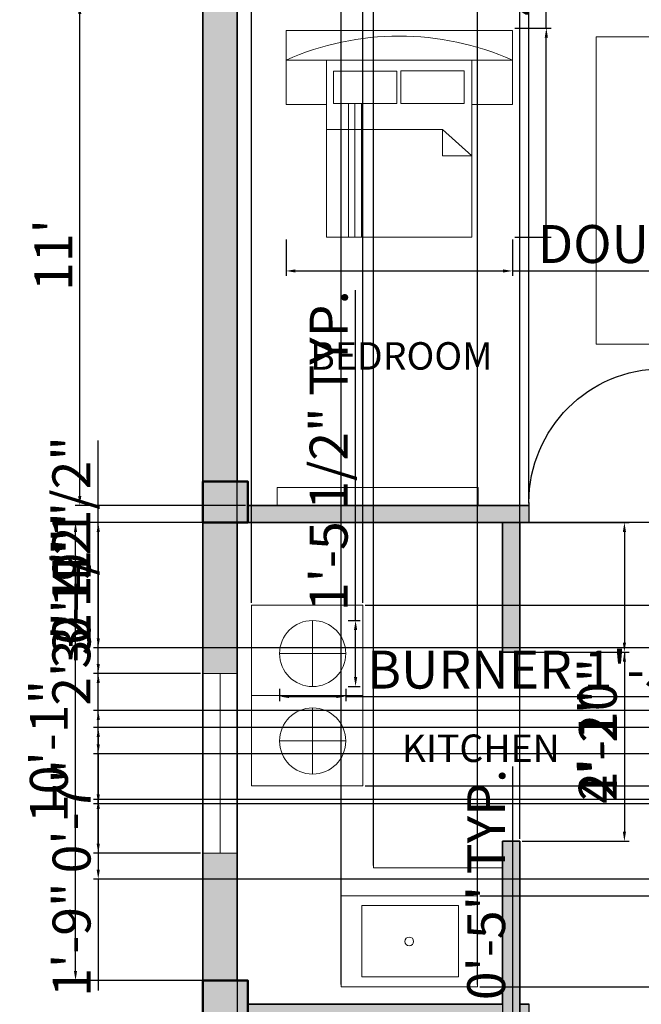
# Model space of a CAD drawing. Units: inches. Extents: x 2312 to 2808, y 1290 to 1909.
# Tile 2 of 5: x 2312 to 2476, y 1503 to 1763. Entities that reach past the tile are written whole.
import ezdxf

# ---------------------------------------------------------------- set-up
doc = ezdxf.new("R2010")
doc.units = ezdxf.units.IN
for name, color, linetype, lineweight in [('A-ANNO-DIMS', 2, 'Continuous', 18), ('A-AREA-IDEN', 7, 'Continuous', 25), ('A-COLS-PATT', 1, 'Continuous', 13), ('A-EQPM', 210, 'Continuous', 18), ('A-FLOR-CASE', 181, 'Continuous', 20), ('A-FLOR-FIXT', 9, 'Continuous', 18), ('A-WALL-PATT', 150, 'Continuous', 13), ('COLUMN', 1, 'Continuous', 50), ('DOOR', 50, 'Continuous', 25), ('FUR', 130, 'Continuous', 18), ('WALL', 7, 'Continuous', 35), ('WINDOW', 70, 'Continuous', 18)]:
    doc.layers.add(name, color=color, linetype=linetype, lineweight=lineweight)
doc.styles.get("Standard").update_dxf_attribs({"font": 'arial.ttf'})
doc.dimstyles.new('ISO-25', dxfattribs={"dimtxt": 10, "dimasz": 2.5, "dimexe": 1.25, "dimexo": 0.625, "dimtad": 1, "dimdec": 0, "dimlunit": 4, "dimtxsty": 'Standard', "dimcen": 2.5, "dimadec": 0, "dimazin": 0, "dimtfac": 1, "dimtdec": 0, "dimtmove": 0, "dimatfit": 3, "dimfxl": 1, "dimarcsym": 0})

# ---------------------------------------------------------------- blocks, each defined once
blk = doc.blocks.new('*U2')
for p, q in [((0, 0), (0, -6)), ((40, 0), (40, -6))]:
    blk.add_line(p, q)
blk.add_lwpolyline([(0, 0), (0, 40), (1.75, 40), (1.75, 0)], close=True)
blk.add_arc((0, 0), 40, 0, 90)
blk = doc.blocks.new('*D20')
at = {"layer": 'A-ANNO-DIMS', "color": 0, "lineweight": -2, "transparency": 16777216}
for p, q in [((2368.81, 1630.22), (2325.59, 1630.22)), ((2326.84, 1511.99), (2326.84, 1627.72)), ((2368.81, 1509.49), (2325.59, 1509.49))]:
    blk.add_line(p, q, dxfattribs=at)
at = {"layer": 'A-ANNO-DIMS', "color": 0, "transparency": 16777216}
for points in [[(2326.42, 1627.72), (2327.25, 1627.72), (2326.84, 1630.22)], [(2326.42, 1511.99), (2327.25, 1511.99), (2326.84, 1509.49)]]:
    blk.add_solid(points, dxfattribs=at)
at = {"layer": 'Defpoints', "color": 0, "transparency": 16777216}
for p in [(2326.84, 1630.22), (2369.43, 1630.22), (2369.43, 1509.49)]:
    blk.add_point(p, dxfattribs=at)
at = {"layer": 'A-ANNO-DIMS', "color": 0, "transparency": 16777216, "insert": (2321.11, 1569.86), "char_height": 10, "attachment_point": 5, "rotation": 90}
blk.add_mtext('10\'-1"', dxfattribs=at)
blk = doc.blocks.new('*D21')
at = {"layer": 'A-ANNO-DIMS', "color": 0, "lineweight": -2, "transparency": 16777216}
for p, q in [((2371.65, 1766.72), (2326.71, 1766.72)), ((2327.96, 1637.22), (2327.96, 1764.22)), ((2371.65, 1634.72), (2326.71, 1634.72))]:
    blk.add_line(p, q, dxfattribs=at)
at = {"layer": 'A-ANNO-DIMS', "color": 0, "transparency": 16777216}
for points in [[(2327.54, 1764.22), (2328.38, 1764.22), (2327.96, 1766.72)], [(2327.54, 1637.22), (2328.38, 1637.22), (2327.96, 1634.72)]]:
    blk.add_solid(points, dxfattribs=at)
at = {"layer": 'Defpoints', "color": 0, "transparency": 16777216}
for p in [(2327.96, 1766.72), (2372.28, 1766.72), (2372.28, 1634.72)]:
    blk.add_point(p, dxfattribs=at)
at = {"layer": 'A-ANNO-DIMS', "color": 0, "transparency": 16777216, "insert": (2322.31, 1700.72), "char_height": 10, "attachment_point": 5, "rotation": 90}
blk.add_mtext("11'", dxfattribs=at)
blk = doc.blocks.new('BED-DOUBLE')
for p, q in [((0, 46.6), (0, 54.42)), ((0, 54.42), (59.67, 54.42)), ((59.67, 54.42), (59.67, 46.6)), ((16.43, 35.15), (16.43, 0)), ((18.15, 35.15), (18.15, 0)), ((19.9, 35.15), (19.9, 0)), ((10.68, 28.37), (10.68, 28.37)), ((10.68, 28.37), (41.23, 28.37)), ((41.23, 28.37), (41.23, 21.43)), ((48.99, 21.43), (41.23, 28.37)), ((41.23, 21.43), (48.99, 21.43))]:
    blk.add_line(p, q)
for points in [[(10.68, 46.6), (0, 46.6), (0, 34.89), (10.68, 34.89)], [(10.68, 46.6), (48.99, 46.6), (48.99, 0), (10.68, 0)], [(59.67, 46.6), (48.99, 46.6), (48.99, 34.89), (59.67, 34.89)], [(12.51, 43.74), (29.18, 43.74), (29.18, 35.15), (12.51, 35.15)], [(30.28, 43.78), (46.95, 43.78), (46.95, 35.19), (30.28, 35.19)]]:
    blk.add_lwpolyline(points, close=True)
blk.add_arc((29.84, -20.26), 73.22, 65.9516, 114.0484)
blk = doc.blocks.new('BEDROOM-STORAGE')
blk.add_lwpolyline([(18.34, 80.97), (0, 80.97), (0, 0), (18.34, 0)], close=True)
blk = doc.blocks.new('BEDROOM-WALL-UNIT')
blk.add_lwpolyline([(0, 0), (52.94, 0), (52.94, 4.76), (0, 4.76)], close=True)
blk = doc.blocks.new('COOKTOP-BURNER')
for p, q in [((8.7, 8.71), (8.7, 17.41)), ((8.7, 17.41), (8.7, 0)), ((0, 8.71), (17.41, 8.71)), ((17.41, 8.71), (8.7, 8.71))]:
    blk.add_line(p, q)
blk.add_circle((8.7, 8.71), 8.71)
blk = doc.blocks.new('*D29')
at = {"layer": 'A-ANNO-DIMS', "color": 0, "lineweight": -2, "transparency": 16777216}
for p, q in [((2382.33, 1704.84), (2382.33, 1695.26)), ((2442, 1704.84), (2442, 1695.26)), ((2384.83, 1696.51), (2439.5, 1696.51)), ((2442, 1696.51), (2631.22, 1696.51))]:
    blk.add_line(p, q, dxfattribs=at)
at = {"layer": 'A-ANNO-DIMS', "color": 0, "transparency": 16777216}
for points in [[(2384.83, 1696.93), (2384.83, 1696.09), (2382.33, 1696.51)], [(2439.5, 1696.93), (2439.5, 1696.09), (2442, 1696.51)]]:
    blk.add_solid(points, dxfattribs=at)
at = {"layer": 'Defpoints', "color": 0, "transparency": 16777216}
for p in [(2382.33, 1705.46), (2442, 1705.46), (2442, 1696.51)]:
    blk.add_point(p, dxfattribs=at)
at = {"layer": 'A-ANNO-DIMS', "color": 0, "transparency": 16777216, "insert": (2537.86, 1702.31), "char_height": 10, "attachment_point": 5}
blk.add_mtext('DOUBLE BED 4\'-11 1/2" TYP.', dxfattribs=at)
blk = doc.blocks.new('*D30')
at = {"layer": 'A-ANNO-DIMS', "color": 0, "lineweight": -2, "transparency": 16777216}
for p, q in [((2450.95, 1760.54), (2450.95, 1825.65)), ((2442.63, 1760.54), (2452.2, 1760.54)), ((2450.95, 1707.96), (2450.95, 1758.04)), ((2442.63, 1705.46), (2452.2, 1705.46))]:
    blk.add_line(p, q, dxfattribs=at)
at = {"layer": 'A-ANNO-DIMS', "color": 0, "transparency": 16777216}
for points in [[(2450.54, 1758.04), (2451.37, 1758.04), (2450.95, 1760.54)], [(2450.54, 1707.96), (2451.37, 1707.96), (2450.95, 1705.46)]]:
    blk.add_solid(points, dxfattribs=at)
at = {"layer": 'Defpoints', "color": 0, "transparency": 16777216}
for p in [(2442, 1760.54), (2450.95, 1760.54), (2442, 1705.46)]:
    blk.add_point(p, dxfattribs=at)
at = {"layer": 'A-ANNO-DIMS', "color": 0, "transparency": 16777216, "insert": (2445.32, 1794.34), "char_height": 10, "attachment_point": 5, "rotation": 90}
blk.add_mtext('4\'-7" TYP.', dxfattribs=at)
blk = doc.blocks.new('*D33')
at = {"layer": 'A-ANNO-DIMS', "color": 0, "lineweight": -2, "transparency": 16777216}
for p, q in [((2381.24, 1493.33), (2381.24, 1484.77)), ((2434.18, 1493.33), (2434.18, 1484.77)), ((2383.74, 1486.02), (2431.68, 1486.02)), ((2434.18, 1486.02), (2577.69, 1486.02))]:
    blk.add_line(p, q, dxfattribs=at)
at = {"layer": 'A-ANNO-DIMS', "color": 0, "transparency": 16777216}
for points in [[(2383.74, 1486.43), (2383.74, 1485.6), (2381.24, 1486.02)], [(2431.68, 1486.43), (2431.68, 1485.6), (2434.18, 1486.02)]]:
    blk.add_solid(points, dxfattribs=at)
at = {"layer": 'Defpoints', "color": 0, "transparency": 16777216}
for p in [(2381.24, 1493.96), (2434.18, 1493.96), (2434.18, 1486.02)]:
    blk.add_point(p, dxfattribs=at)
at = {"layer": 'A-ANNO-DIMS', "color": 0, "transparency": 16777216, "insert": (2507.19, 1491.73), "char_height": 10, "attachment_point": 5}
blk.add_mtext('WALL UNIT 4\'-5" TYP.', dxfattribs=at)
blk = doc.blocks.new('*D34')
at = {"layer": 'A-ANNO-DIMS', "color": 0, "lineweight": -2, "transparency": 16777216}
for p, q in [((2442.12, 1501.22), (2442.12, 1565.92)), ((2434.81, 1498.72), (2443.37, 1498.72)), ((2442.12, 1493.96), (2442.12, 1498.72)), ((2434.81, 1493.96), (2443.37, 1493.96)), ((2442.12, 1491.46), (2442.12, 1488.96))]:
    blk.add_line(p, q, dxfattribs=at)
at = {"layer": 'A-ANNO-DIMS', "color": 0, "transparency": 16777216}
for points in [[(2441.7, 1501.22), (2442.54, 1501.22), (2442.12, 1498.72)], [(2441.7, 1491.46), (2442.54, 1491.46), (2442.12, 1493.96)]]:
    blk.add_solid(points, dxfattribs=at)
at = {"layer": 'Defpoints', "color": 0, "transparency": 16777216}
for p in [(2434.18, 1498.72), (2442.12, 1498.72), (2434.18, 1493.96)]:
    blk.add_point(p, dxfattribs=at)
at = {"layer": 'A-ANNO-DIMS', "color": 0, "transparency": 16777216, "insert": (2436.39, 1534.82), "char_height": 10, "attachment_point": 5, "rotation": 90}
blk.add_mtext('0\'-5" TYP.', dxfattribs=at)
blk = doc.blocks.new('*D37')
at = {"layer": 'A-ANNO-DIMS', "color": 0, "lineweight": -2, "transparency": 16777216}
for p, q in [((2380.65, 1586.33), (2380.65, 1583.1)), ((2398.06, 1586.33), (2398.06, 1583.1)), ((2383.15, 1584.35), (2395.56, 1584.35)), ((2398.06, 1584.35), (2548.49, 1584.35))]:
    blk.add_line(p, q, dxfattribs=at)
at = {"layer": 'A-ANNO-DIMS', "color": 0, "transparency": 16777216}
for points in [[(2383.15, 1584.76), (2383.15, 1583.93), (2380.65, 1584.35)], [(2395.56, 1584.76), (2395.56, 1583.93), (2398.06, 1584.35)]]:
    blk.add_solid(points, dxfattribs=at)
at = {"layer": 'Defpoints', "color": 0, "transparency": 16777216}
for p in [(2380.65, 1586.96), (2398.06, 1586.96), (2398.06, 1584.35)]:
    blk.add_point(p, dxfattribs=at)
at = {"layer": 'A-ANNO-DIMS', "color": 0, "transparency": 16777216, "insert": (2474.53, 1590.14), "char_height": 10, "attachment_point": 5}
blk.add_mtext('BURNER 1\'-5 1/2" TYP.', dxfattribs=at)
blk = doc.blocks.new('*D38')
at = {"layer": 'A-ANNO-DIMS', "color": 0, "lineweight": -2, "transparency": 16777216}
for p, q in [((2400.67, 1604.37), (2400.67, 1691.43)), ((2398.68, 1604.37), (2401.92, 1604.37)), ((2400.67, 1589.46), (2400.67, 1601.87)), ((2398.68, 1586.96), (2401.92, 1586.96))]:
    blk.add_line(p, q, dxfattribs=at)
at = {"layer": 'A-ANNO-DIMS', "color": 0, "transparency": 16777216}
for points in [[(2400.25, 1601.87), (2401.09, 1601.87), (2400.67, 1604.37)], [(2400.25, 1589.46), (2401.09, 1589.46), (2400.67, 1586.96)]]:
    blk.add_solid(points, dxfattribs=at)
at = {"layer": 'Defpoints', "color": 0, "transparency": 16777216}
for p in [(2398.06, 1604.37), (2400.67, 1604.37), (2398.06, 1586.96)]:
    blk.add_point(p, dxfattribs=at)
at = {"layer": 'A-ANNO-DIMS', "color": 0, "transparency": 16777216, "insert": (2394.87, 1649.15), "char_height": 10, "attachment_point": 5, "rotation": 90}
blk.add_mtext('1\'-5 1/2" TYP.', dxfattribs=at)
blk = doc.blocks.new('*D40')
at = {"layer": 'A-ANNO-DIMS', "color": 0, "lineweight": -2, "transparency": 16777216}
for p, q in [((2439.43, 1545.58), (2439.43, 1326.46)), ((2369.43, 1542.44), (2369.43, 1326.46)), ((2371.93, 1327.71), (2436.93, 1327.71))]:
    blk.add_line(p, q, dxfattribs=at)
at = {"layer": 'A-ANNO-DIMS', "color": 0, "transparency": 16777216}
for points in [[(2371.93, 1328.13), (2371.93, 1327.3), (2369.43, 1327.71)], [(2436.93, 1328.13), (2436.93, 1327.3), (2439.43, 1327.71)]]:
    blk.add_solid(points, dxfattribs=at)
at = {"layer": 'Defpoints', "color": 0, "transparency": 16777216}
for p in [(2439.43, 1546.2), (2369.43, 1543.07), (2439.43, 1327.71)]:
    blk.add_point(p, dxfattribs=at)
at = {"layer": 'A-ANNO-DIMS', "color": 0, "transparency": 16777216, "insert": (2404.43, 1333.44), "char_height": 10, "attachment_point": 5}
blk.add_mtext('5\'-10"', dxfattribs=at)
blk = doc.blocks.new('*D41')
at = {"layer": 'A-ANNO-DIMS', "color": 0, "lineweight": -2, "transparency": 16777216}
for p, q in [((2443.93, 1546.83), (2443.93, 1804.57)), ((2482.43, 1510.12), (2482.43, 1804.57)), ((2446.43, 1803.32), (2479.93, 1803.32)), ((2482.43, 1803.32), (2536.06, 1803.32))]:
    blk.add_line(p, q, dxfattribs=at)
at = {"layer": 'A-ANNO-DIMS', "color": 0, "transparency": 16777216}
for points in [[(2446.43, 1803.73), (2446.43, 1802.9), (2443.93, 1803.32)], [(2479.93, 1803.73), (2479.93, 1802.9), (2482.43, 1803.32)]]:
    blk.add_solid(points, dxfattribs=at)
at = {"layer": 'Defpoints', "color": 0, "transparency": 16777216}
for p in [(2482.43, 1803.32), (2443.93, 1546.2), (2482.43, 1509.49)]:
    blk.add_point(p, dxfattribs=at)
at = {"layer": 'A-ANNO-DIMS', "color": 0, "transparency": 16777216, "insert": (2510.5, 1809.12), "char_height": 10, "attachment_point": 5}
blk.add_mtext('3\'-2 1/2"', dxfattribs=at)
blk = doc.blocks.new('*D50')
at = {"layer": 'A-ANNO-DIMS', "color": 0, "lineweight": -2, "transparency": 16777216}
for p, q in [((2446.36, 1635.34), (2446.36, 1804.57)), ((2482.43, 1635.34), (2482.43, 1804.57)), ((2448.86, 1803.32), (2479.93, 1803.32))]:
    blk.add_line(p, q, dxfattribs=at)
at = {"layer": 'A-ANNO-DIMS', "color": 0, "transparency": 16777216}
for points in [[(2448.86, 1803.73), (2448.86, 1802.9), (2446.36, 1803.32)], [(2479.93, 1803.73), (2479.93, 1802.9), (2482.43, 1803.32)]]:
    blk.add_solid(points, dxfattribs=at)
at = {"layer": 'Defpoints', "color": 0, "transparency": 16777216}
for p in [(2482.43, 1803.32), (2446.36, 1634.72), (2482.43, 1634.72)]:
    blk.add_point(p, dxfattribs=at)
at = {"layer": 'A-ANNO-DIMS', "color": 0, "transparency": 16777216, "insert": (2464.4, 1809.05), "char_height": 10, "attachment_point": 5}
blk.add_mtext('3\'-0"', dxfattribs=at)
blk = doc.blocks.new('*D52')
at = {"layer": 'A-ANNO-DIMS', "color": 0, "lineweight": -2, "transparency": 16777216}
for p, q in [((2332.83, 1590.4), (2332.83, 1651.79)), ((2359.81, 1590.4), (2331.58, 1590.4)), ((2332.83, 1545.57), (2332.83, 1587.9)), ((2359.81, 1543.07), (2331.58, 1543.07))]:
    blk.add_line(p, q, dxfattribs=at)
at = {"layer": 'A-ANNO-DIMS', "color": 0, "transparency": 16777216}
for points in [[(2332.42, 1587.9), (2333.25, 1587.9), (2332.83, 1590.4)], [(2332.42, 1545.57), (2333.25, 1545.57), (2332.83, 1543.07)]]:
    blk.add_solid(points, dxfattribs=at)
at = {"layer": 'Defpoints', "color": 0, "transparency": 16777216}
for p in [(2332.83, 1590.4), (2360.43, 1590.4), (2360.43, 1543.07)]:
    blk.add_point(p, dxfattribs=at)
at = {"layer": 'A-ANNO-DIMS', "color": 0, "transparency": 16777216, "insert": (2327.04, 1622.35), "char_height": 10, "attachment_point": 5, "rotation": 90}
blk.add_mtext('3\'-11 1/2"', dxfattribs=at)
blk = doc.blocks.new('*D53')
at = {"layer": 'A-ANNO-DIMS', "color": 0, "lineweight": -2, "transparency": 16777216}
for p, q in [((2369.43, 1543.69), (2369.43, 1804.57)), ((2405.43, 1539.84), (2405.43, 1804.57)), ((2371.93, 1803.32), (2402.93, 1803.32))]:
    blk.add_line(p, q, dxfattribs=at)
at = {"layer": 'A-ANNO-DIMS', "color": 0, "transparency": 16777216}
for points in [[(2371.93, 1803.73), (2371.93, 1802.9), (2369.43, 1803.32)], [(2402.93, 1803.73), (2402.93, 1802.9), (2405.43, 1803.32)]]:
    blk.add_solid(points, dxfattribs=at)
at = {"layer": 'Defpoints', "color": 0, "transparency": 16777216}
for p in [(2405.43, 1803.32), (2369.43, 1543.07), (2405.43, 1539.22)]:
    blk.add_point(p, dxfattribs=at)
at = {"layer": 'A-ANNO-DIMS', "color": 0, "transparency": 16777216, "insert": (2387.43, 1809.05), "char_height": 10, "attachment_point": 5}
blk.add_mtext('3\'-0"', dxfattribs=at)
blk = doc.blocks.new('*D55')
at = {"layer": 'A-ANNO-DIMS', "color": 0, "lineweight": -2, "transparency": 16777216}
for p, q in [((2332.83, 1580.62), (2332.83, 1634.43)), ((2544.39, 1580.62), (2331.58, 1580.62)), ((2332.83, 1558.54), (2332.83, 1578.12)), ((2544.39, 1556.04), (2331.58, 1556.04))]:
    blk.add_line(p, q, dxfattribs=at)
at = {"layer": 'A-ANNO-DIMS', "color": 0, "transparency": 16777216}
for points in [[(2332.42, 1578.12), (2333.25, 1578.12), (2332.83, 1580.62)], [(2332.42, 1558.54), (2333.25, 1558.54), (2332.83, 1556.04)]]:
    blk.add_solid(points, dxfattribs=at)
at = {"layer": 'Defpoints', "color": 0, "transparency": 16777216}
for p in [(2332.83, 1580.62), (2545.01, 1580.62), (2545.01, 1556.04)]:
    blk.add_point(p, dxfattribs=at)
at = {"layer": 'A-ANNO-DIMS', "color": 0, "transparency": 16777216, "insert": (2327.04, 1608.77), "char_height": 10, "attachment_point": 5, "rotation": 90}
blk.add_mtext('2\'-0 1/2"', dxfattribs=at)
blk = doc.blocks.new('*D59')
at = {"layer": 'A-ANNO-DIMS', "color": 0, "lineweight": -2, "transparency": 16777216}
for p, q in [((2359.81, 1630.22), (2331.58, 1630.22)), ((2332.83, 1592.9), (2332.83, 1627.72)), ((2359.81, 1590.4), (2331.58, 1590.4))]:
    blk.add_line(p, q, dxfattribs=at)
at = {"layer": 'A-ANNO-DIMS', "color": 0, "transparency": 16777216}
for points in [[(2332.42, 1627.72), (2333.25, 1627.72), (2332.83, 1630.22)], [(2332.42, 1592.9), (2333.25, 1592.9), (2332.83, 1590.4)]]:
    blk.add_solid(points, dxfattribs=at)
at = {"layer": 'Defpoints', "color": 0, "transparency": 16777216}
for p in [(2332.83, 1630.22), (2360.43, 1630.22), (2360.43, 1590.4)]:
    blk.add_point(p, dxfattribs=at)
at = {"layer": 'A-ANNO-DIMS', "color": 0, "transparency": 16777216, "insert": (2327.1, 1610.31), "char_height": 10, "attachment_point": 5, "rotation": 90}
blk.add_mtext('3\'-4"', dxfattribs=at)
blk = doc.blocks.new('*D62')
at = {"layer": 'A-ANNO-DIMS', "color": 0, "lineweight": -2, "transparency": 16777216}
for p, q in [((2396.83, 1508.42), (2396.83, 1804.57)), ((2432.83, 1508.42), (2432.83, 1804.57)), ((2399.33, 1803.32), (2430.33, 1803.32))]:
    blk.add_line(p, q, dxfattribs=at)
at = {"layer": 'A-ANNO-DIMS', "color": 0, "transparency": 16777216}
for points in [[(2399.33, 1803.73), (2399.33, 1802.9), (2396.83, 1803.32)], [(2430.33, 1803.73), (2430.33, 1802.9), (2432.83, 1803.32)]]:
    blk.add_solid(points, dxfattribs=at)
at = {"layer": 'Defpoints', "color": 0, "transparency": 16777216}
for p in [(2432.83, 1803.32), (2396.83, 1507.8), (2432.83, 1507.8)]:
    blk.add_point(p, dxfattribs=at)
at = {"layer": 'A-ANNO-DIMS', "color": 0, "transparency": 16777216, "insert": (2414.83, 1809.05), "char_height": 10, "attachment_point": 5}
blk.add_mtext('3\'-0"', dxfattribs=at)
blk = doc.blocks.new('*D63')
at = {"layer": 'A-ANNO-DIMS', "color": 0, "lineweight": -2, "transparency": 16777216}
for p, q in [((2799.03, 1531.79), (2799.03, 1562.3)), ((2433.46, 1531.79), (2800.28, 1531.79)), ((2799.03, 1510.3), (2799.03, 1529.29)), ((2433.46, 1507.8), (2800.28, 1507.8))]:
    blk.add_line(p, q, dxfattribs=at)
at = {"layer": 'A-ANNO-DIMS', "color": 0, "transparency": 16777216}
for points in [[(2798.62, 1529.29), (2799.45, 1529.29), (2799.03, 1531.79)], [(2798.62, 1510.3), (2799.45, 1510.3), (2799.03, 1507.8)]]:
    blk.add_solid(points, dxfattribs=at)
at = {"layer": 'Defpoints', "color": 0, "transparency": 16777216}
for p in [(2432.83, 1531.79), (2799.03, 1531.79), (2432.83, 1507.8)]:
    blk.add_point(p, dxfattribs=at)
at = {"layer": 'A-ANNO-DIMS', "color": 0, "transparency": 16777216, "insert": (2793.3, 1548.3), "char_height": 10, "attachment_point": 5, "rotation": 90}
blk.add_mtext('2\'-0"', dxfattribs=at)
blk = doc.blocks.new('*D65')
at = {"layer": 'A-ANNO-DIMS', "color": 0, "lineweight": -2, "transparency": 16777216}
for p, q in [((2710.81, 1557.21), (2331.58, 1557.21)), ((2332.83, 1554.71), (2332.83, 1538.71)), ((2710.81, 1536.21), (2331.58, 1536.21)), ((2332.83, 1536.21), (2332.83, 1506.82))]:
    blk.add_line(p, q, dxfattribs=at)
at = {"layer": 'A-ANNO-DIMS', "color": 0, "transparency": 16777216}
for points in [[(2332.42, 1554.71), (2333.25, 1554.71), (2332.83, 1557.21)], [(2332.42, 1538.71), (2333.25, 1538.71), (2332.83, 1536.21)]]:
    blk.add_solid(points, dxfattribs=at)
at = {"layer": 'Defpoints', "color": 0, "transparency": 16777216}
for p in [(2711.43, 1557.21), (2332.83, 1536.21), (2711.43, 1536.21)]:
    blk.add_point(p, dxfattribs=at)
at = {"layer": 'A-ANNO-DIMS', "color": 0, "transparency": 16777216, "insert": (2327.1, 1520.27), "char_height": 10, "attachment_point": 5, "rotation": 90}
blk.add_mtext('1\'-9"', dxfattribs=at)
blk = doc.blocks.new('*D72')
at = {"layer": 'A-ANNO-DIMS', "color": 0, "lineweight": -2, "transparency": 16777216}
for p, q in [((2702.81, 1576.18), (2331.58, 1576.18)), ((2332.83, 1573.68), (2332.83, 1571.72)), ((2710.81, 1569.22), (2331.58, 1569.22)), ((2332.83, 1569.22), (2332.83, 1538.88))]:
    blk.add_line(p, q, dxfattribs=at)
at = {"layer": 'A-ANNO-DIMS', "color": 0, "transparency": 16777216}
for points in [[(2332.42, 1573.68), (2333.25, 1573.68), (2332.83, 1576.18)], [(2332.42, 1571.72), (2333.25, 1571.72), (2332.83, 1569.22)]]:
    blk.add_solid(points, dxfattribs=at)
at = {"layer": 'Defpoints', "color": 0, "transparency": 16777216}
for p in [(2703.43, 1576.18), (2332.83, 1569.22), (2711.43, 1569.22)]:
    blk.add_point(p, dxfattribs=at)
at = {"layer": 'A-ANNO-DIMS', "color": 0, "transparency": 16777216, "insert": (2327.1, 1552.8), "char_height": 10, "attachment_point": 5, "rotation": 90}
blk.add_mtext('0\'-7"', dxfattribs=at)
blk = doc.blocks.new('*D73')
at = {"layer": 'A-ANNO-DIMS', "color": 0, "lineweight": -2, "transparency": 16777216}
for p, q in [((2373.27, 1609.07), (2373.27, 1804.57)), ((2402.58, 1609.07), (2402.58, 1804.57)), ((2375.77, 1803.32), (2400.08, 1803.32)), ((2402.58, 1803.32), (2456.39, 1803.32))]:
    blk.add_line(p, q, dxfattribs=at)
at = {"layer": 'A-ANNO-DIMS', "color": 0, "transparency": 16777216}
for points in [[(2375.77, 1803.73), (2375.77, 1802.9), (2373.27, 1803.32)], [(2400.08, 1803.73), (2400.08, 1802.9), (2402.58, 1803.32)]]:
    blk.add_solid(points, dxfattribs=at)
at = {"layer": 'Defpoints', "color": 0, "transparency": 16777216}
for p in [(2402.58, 1803.32), (2373.27, 1608.44), (2402.58, 1608.44)]:
    blk.add_point(p, dxfattribs=at)
at = {"layer": 'A-ANNO-DIMS', "color": 0, "transparency": 16777216, "insert": (2430.74, 1809.11), "char_height": 10, "attachment_point": 5}
blk.add_mtext('2\'-5 1/2"', dxfattribs=at)
blk = doc.blocks.new('*D74')
at = {"layer": 'A-ANNO-DIMS', "color": 0, "lineweight": -2, "transparency": 16777216}
for p, q in [((2799.03, 1608.44), (2799.03, 1669.84)), ((2403.21, 1608.44), (2800.28, 1608.44)), ((2799.03, 1563.31), (2799.03, 1605.94)), ((2403.21, 1560.81), (2800.28, 1560.81))]:
    blk.add_line(p, q, dxfattribs=at)
at = {"layer": 'A-ANNO-DIMS', "color": 0, "transparency": 16777216}
for points in [[(2798.62, 1605.94), (2799.45, 1605.94), (2799.03, 1608.44)], [(2798.62, 1563.31), (2799.45, 1563.31), (2799.03, 1560.81)]]:
    blk.add_solid(points, dxfattribs=at)
at = {"layer": 'Defpoints', "color": 0, "transparency": 16777216}
for p in [(2402.58, 1608.44), (2799.03, 1608.44), (2402.58, 1560.81)]:
    blk.add_point(p, dxfattribs=at)
at = {"layer": 'A-ANNO-DIMS', "color": 0, "transparency": 16777216, "insert": (2793.24, 1640.39), "char_height": 10, "attachment_point": 5, "rotation": 90}
blk.add_mtext('3\'-11 1/2"', dxfattribs=at)
blk = doc.blocks.new('*D75')
at = {"layer": 'A-ANNO-DIMS', "color": 0, "lineweight": -2, "transparency": 16777216}
for p, q in [((2641.28, 1630.22), (2331.58, 1630.22)), ((2332.83, 1627.72), (2332.83, 1599.71)), ((2641.28, 1597.21), (2331.58, 1597.21))]:
    blk.add_line(p, q, dxfattribs=at)
at = {"layer": 'A-ANNO-DIMS', "color": 0, "transparency": 16777216}
for points in [[(2332.42, 1627.72), (2333.25, 1627.72), (2332.83, 1630.22)], [(2332.42, 1599.71), (2333.25, 1599.71), (2332.83, 1597.21)]]:
    blk.add_solid(points, dxfattribs=at)
at = {"layer": 'Defpoints', "color": 0, "transparency": 16777216}
for p in [(2641.91, 1630.22), (2332.83, 1597.21), (2641.91, 1597.21)]:
    blk.add_point(p, dxfattribs=at)
at = {"layer": 'A-ANNO-DIMS', "color": 0, "transparency": 16777216, "insert": (2327.1, 1613.71), "char_height": 10, "attachment_point": 5, "rotation": 90}
blk.add_mtext('2\'-9"', dxfattribs=at)
blk = doc.blocks.new('*D76')
at = {"layer": 'A-ANNO-DIMS', "color": 0, "lineweight": -2, "transparency": 16777216}
for p, q in [((2444.56, 1596.05), (2472.78, 1596.05)), ((2471.53, 1593.55), (2471.53, 1548.7)), ((2444.56, 1546.2), (2472.78, 1546.2))]:
    blk.add_line(p, q, dxfattribs=at)
at = {"layer": 'A-ANNO-DIMS', "color": 0, "transparency": 16777216}
for points in [[(2471.12, 1593.55), (2471.95, 1593.55), (2471.53, 1596.05)], [(2471.12, 1548.7), (2471.95, 1548.7), (2471.53, 1546.2)]]:
    blk.add_solid(points, dxfattribs=at)
at = {"layer": 'Defpoints', "color": 0, "transparency": 16777216}
for p in [(2443.93, 1596.05), (2443.93, 1546.2), (2471.53, 1546.2)]:
    blk.add_point(p, dxfattribs=at)
at = {"layer": 'A-ANNO-DIMS', "color": 0, "transparency": 16777216, "insert": (2465.89, 1571.13), "char_height": 10, "attachment_point": 5, "rotation": 90}
blk.add_mtext('4\'-2"', dxfattribs=at)
blk = doc.blocks.new('*D77')
at = {"layer": 'A-ANNO-DIMS', "color": 0, "lineweight": -2, "transparency": 16777216}
for p, q in [((2444.56, 1630.22), (2472.78, 1630.22)), ((2471.53, 1627.72), (2471.53, 1598.55)), ((2444.56, 1596.05), (2472.78, 1596.05)), ((2471.53, 1596.05), (2471.53, 1557.78))]:
    blk.add_line(p, q, dxfattribs=at)
at = {"layer": 'A-ANNO-DIMS', "color": 0, "transparency": 16777216}
for points in [[(2471.12, 1627.72), (2471.95, 1627.72), (2471.53, 1630.22)], [(2471.12, 1598.55), (2471.95, 1598.55), (2471.53, 1596.05)]]:
    blk.add_solid(points, dxfattribs=at)
at = {"layer": 'Defpoints', "color": 0, "transparency": 16777216}
for p in [(2443.93, 1630.22), (2443.93, 1596.05), (2471.53, 1596.05)]:
    blk.add_point(p, dxfattribs=at)
at = {"layer": 'A-ANNO-DIMS', "color": 0, "transparency": 16777216, "insert": (2465.8, 1575.67), "char_height": 10, "attachment_point": 5, "rotation": 90}
blk.add_mtext('2\'-10"', dxfattribs=at)

msp = doc.modelspace()

# ---------------------------------------------------------------- hatches: boundary and pattern name
at = {"layer": 'A-COLS-PATT'}
h = msp.add_hatch(color=256, dxfattribs=at)
h.dxf.hatch_style = 1
h.paths.add_polyline_path([(2372.28, 1775.72), (2360.43, 1775.72), (2360.43, 1764.94), (2372.28, 1764.94)])
h.paths.add_polyline_path([(2486.97, 1775.72), (2475.12, 1775.72), (2475.12, 1764.94), (2486.93, 1764.94), (2486.93, 1766.72)])
h.paths.add_polyline_path([(2610.92, 1775.72), (2599.07, 1775.72), (2599.07, 1766.72), (2599.11, 1766.72), (2599.11, 1764.94), (2610.92, 1764.94)])
h.paths.add_polyline_path([(2720.43, 1775.72), (2708.59, 1775.72), (2708.59, 1764.94), (2720.43, 1764.94)])
h.paths.add_polyline_path([(2723.28, 1640.11), (2711.43, 1640.11), (2711.43, 1629.34), (2723.28, 1629.34)])
h.paths.add_polyline_path([(2603.61, 1640.99), (2592.09, 1640.99), (2592.09, 1630.22), (2603.93, 1630.22), (2603.93, 1634.72), (2603.61, 1634.72)])
h.paths.add_polyline_path([(2494.28, 1640.99), (2482.43, 1640.99), (2482.43, 1630.22), (2494.28, 1630.22)])
h.paths.add_polyline_path([(2372.28, 1640.99), (2360.43, 1640.99), (2360.43, 1630.22), (2372.28, 1630.22)])
h.paths.add_polyline_path([(2372.28, 1509.49), (2360.43, 1509.49), (2360.43, 1498.72), (2372.28, 1498.72)])
h.paths.add_polyline_path([(2494.28, 1509.49), (2482.43, 1509.49), (2482.43, 1498.72), (2494.28, 1498.72)])
h.paths.add_polyline_path([(2603.93, 1509.49), (2592.09, 1509.49), (2592.09, 1498.72), (2603.93, 1498.72)])
h.paths.add_polyline_path([(2723.28, 1509.26), (2711.43, 1509.26), (2711.43, 1498.48), (2723.28, 1498.48)])
h.paths.add_polyline_path([(2720.43, 1378.49), (2708.59, 1378.49), (2708.59, 1367.72), (2720.43, 1367.72)])
h.paths.add_polyline_path([(2610.2, 1378.49), (2598.36, 1378.49), (2598.36, 1367.72), (2610.2, 1367.72)])
h.paths.add_polyline_path([(2486.94, 1376.72), (2486.93, 1376.72), (2486.93, 1378.49), (2475.1, 1378.49), (2475.1, 1367.72), (2486.94, 1367.72)])
h.paths.add_polyline_path([(2372.28, 1378.49), (2360.43, 1378.49), (2360.43, 1367.72), (2372.28, 1367.72)])
at = {"layer": 'A-WALL-PATT'}
h = msp.add_hatch(color=256, dxfattribs=at)
h.dxf.hatch_style = 1
h.paths.add_polyline_path([(2369.43, 1764.94), (2360.43, 1764.94), (2360.43, 1640.99), (2369.43, 1640.99)])
h.paths.add_polyline_path([(2720.43, 1764.94), (2711.43, 1764.94), (2711.43, 1640.11), (2720.43, 1640.11)])
h.paths.add_polyline_path([(2552.09, 1634.72), (2494.28, 1634.72), (2494.28, 1630.22), (2552.09, 1630.22)])
h.paths.add_polyline_path([(2446.36, 1634.72), (2372.28, 1634.72), (2372.28, 1630.22), (2405.43, 1630.22), (2439.43, 1630.22), (2446.36, 1630.22)])
h.paths.add_polyline_path([(2443.93, 1630.22), (2439.43, 1630.22), (2439.43, 1596.05), (2443.93, 1596.05)])
h.paths.add_polyline_path([(2486.93, 1630.22), (2482.43, 1630.22), (2482.43, 1509.49), (2486.93, 1509.49)])
h.paths.add_polyline_path([(2443.93, 1546.2), (2439.43, 1546.2), (2439.43, 1503.22), (2372.28, 1503.22), (2372.28, 1498.72), (2443.93, 1498.72)])
h.paths.add_polyline_path([(2555.45, 1503.22), (2494.28, 1503.22), (2494.28, 1498.72), (2555.45, 1498.72)])
h.paths.add_polyline_path([(2711.43, 1503.22), (2639.88, 1503.22), (2639.88, 1498.72), (2711.43, 1498.72)])
h.paths.add_polyline_path([(2646.41, 1564.72), (2711.43, 1564.72), (2711.43, 1569.22), (2646.41, 1569.22), (2646.41, 1597.21), (2641.91, 1597.21), (2641.91, 1564.72), (2641.91, 1536.48), (2646.41, 1536.48)])
h.paths.add_polyline_path([(2720.43, 1498.48), (2711.43, 1498.48), (2711.43, 1378.49), (2720.43, 1378.49)])
h.paths.add_polyline_path([(2369.43, 1498.72), (2360.43, 1498.72), (2360.43, 1378.49), (2369.43, 1378.49)])
h.paths.add_polyline_path([(2486.93, 1498.72), (2482.43, 1498.72), (2482.43, 1378.49), (2486.93, 1378.49)])
h.paths.add_polyline_path([(2603.93, 1498.72), (2599.11, 1498.72), (2599.11, 1378.49), (2603.93, 1378.49)])
h.paths.add_polyline_path([(2510.36, 1766.72), (2510.36, 1775.72), (2486.97, 1775.72), (2486.97, 1766.72)])
h.paths.add_polyline_path([(2571.02, 1775.72), (2571.02, 1766.72), (2599.07, 1766.72), (2599.07, 1775.72)])
h.paths.add_polyline_path([(2393.8, 1766.72), (2393.8, 1775.72), (2372.28, 1775.72), (2372.28, 1766.72)])
h.paths.add_polyline_path([(2454.45, 1775.72), (2454.45, 1766.72), (2475.12, 1766.72), (2475.12, 1775.72)])
h.paths.add_polyline_path([(2694.96, 1775.72), (2694.96, 1766.72), (2708.59, 1766.72), (2708.59, 1775.72)])
h.paths.add_polyline_path([(2634.31, 1766.72), (2634.31, 1775.72), (2610.92, 1775.72), (2610.92, 1766.72)])
h.paths.add_polyline_path([(2392.25, 1367.72), (2392.25, 1376.72), (2372.28, 1376.72), (2372.28, 1367.72)])
h.paths.add_polyline_path([(2452.9, 1376.72), (2452.9, 1367.72), (2475.1, 1367.72), (2475.1, 1376.72)])
h.paths.add_polyline_path([(2508.56, 1376.72), (2508.56, 1367.72), (2558.63, 1367.72), (2558.63, 1370.65), (2558.63, 1376.72)])
h.paths.add_polyline_path([(2488.96, 1367.72), (2488.96, 1376.72), (2486.94, 1376.72), (2486.94, 1367.72)])
h.paths.add_polyline_path([(2634.6, 1367.72), (2634.6, 1376.72), (2610.2, 1376.72), (2610.2, 1367.72)])
h.paths.add_polyline_path([(2695.25, 1376.72), (2695.25, 1367.72), (2708.59, 1367.72), (2708.59, 1376.72)])
h.paths.add_polyline_path([(2360.43, 1590.4), (2369.43, 1590.4), (2369.43, 1630.22), (2360.43, 1630.22)])
h.paths.add_polyline_path([(2369.43, 1543.07), (2360.43, 1543.07), (2360.43, 1509.49), (2369.43, 1509.49)])
h.paths.add_polyline_path([(2720.43, 1531.67), (2711.43, 1531.67), (2711.43, 1509.26), (2720.43, 1509.26)])
h.paths.add_polyline_path([(2720.43, 1572.68), (2711.43, 1572.68), (2711.43, 1558.71), (2720.43, 1558.71)])
h.paths.add_polyline_path([(2711.43, 1599.72), (2720.43, 1599.72), (2720.43, 1629.34), (2711.43, 1629.34)])
h = msp.add_hatch(color=256, dxfattribs=at)
h.dxf.hatch_style = 1
h.paths.add_polyline_path([(2446.46, 1503.22), (2443.93, 1503.22), (2443.93, 1498.72), (2446.46, 1498.72)])
h.paths.add_polyline_path([(2482.43, 1503.22), (2481.69, 1503.22), (2481.69, 1498.72), (2482.43, 1498.72)])
h.paths.add_polyline_path([(2592.09, 1503.22), (2590.68, 1503.22), (2590.68, 1498.72), (2592.09, 1498.72)])
h.paths.add_polyline_path([(2604.66, 1503.22), (2603.93, 1503.22), (2603.93, 1498.72), (2604.66, 1498.72)])

# ---------------------------------------------------------------- linework, layer by layer
at = {"layer": 'A-EQPM'}
msp.add_line((2373.27, 1584.62), (2402.58, 1584.62), dxfattribs=at)
msp.add_lwpolyline([(2373.27, 1608.44), (2402.58, 1608.44), (2402.58, 1560.81), (2373.27, 1560.81)], close=True, dxfattribs=at)
at = {"layer": 'A-FLOR-CASE'}
for p, q in [((2369.43, 1630.22), (2405.43, 1630.22)), ((2405.43, 1630.22), (2405.43, 1539.22)), ((2439.43, 1539.22), (2405.43, 1539.22)), ((2439.43, 1503.22), (2439.43, 1539.22))]:
    msp.add_line(p, q, dxfattribs=at)
at = {"layer": 'A-FLOR-FIXT'}
for points in [[(2432.83, 1531.79), (2396.83, 1531.79), (2396.83, 1507.8), (2432.83, 1507.8)], [(2402.31, 1529.27), (2427.82, 1529.27), (2427.82, 1510.48), (2402.31, 1510.48)]]:
    msp.add_lwpolyline(points, close=True, dxfattribs=at)
msp.add_circle((2414.83, 1519.8), 1.15, dxfattribs=at)
at = {"layer": 'COLUMN'}
for points in [[(2360.43, 1640.99), (2372.28, 1640.99), (2372.28, 1630.22), (2360.43, 1630.22)], [(2360.43, 1509.49), (2372.28, 1509.49), (2372.28, 1498.72), (2360.43, 1498.72)]]:
    msp.add_lwpolyline(points, close=True, dxfattribs=at)
at = {"layer": 'WALL'}
for p, q in [((2360.43, 1367.72), (2360.43, 1775.72)), ((2446.36, 1634.72), (2372.28, 1634.72)), ((2369.43, 1630.22), (2439.43, 1630.22)), ((2446.36, 1630.22), (2369.43, 1630.22)), ((2439.43, 1630.22), (2439.43, 1596.05)), ((2443.93, 1630.22), (2443.93, 1596.05)), ((2439.43, 1596.05), (2443.93, 1596.05)), ((2439.43, 1546.2), (2443.93, 1546.2)), ((2439.43, 1546.2), (2439.43, 1503.22)), ((2443.93, 1546.2), (2443.93, 1498.72)), ((2439.43, 1503.22), (2372.28, 1503.22)), ((2443.93, 1503.22), (2446.46, 1503.22))]:
    msp.add_line(p, q, dxfattribs=at)
for points in [[(2720.43, 1498.48), (2720.43, 1367.72), (2360.43, 1367.72), (2360.43, 1775.72), (2720.43, 1775.72), (2720.43, 1640.11)], [(2369.43, 1640.99), (2369.43, 1764.94)], [(2369.43, 1509.49), (2369.43, 1630.22)]]:
    msp.add_lwpolyline(points, dxfattribs=at)
at = {"layer": 'WINDOW'}
msp.add_line((2364.93, 1590.4), (2364.93, 1543.07), dxfattribs=at)
msp.add_lwpolyline([(2360.43, 1590.4), (2369.43, 1590.4), (2369.43, 1543.07), (2360.43, 1543.07)], close=True, dxfattribs=at)

# ---------------------------------------------------------------- block references
at = {"layer": 'A-EQPM'}
for p in [(2380.65, 1586.96), (2380.65, 1563.91)]:
    msp.add_blockref('COOKTOP-BURNER', p, dxfattribs=at)
at = {"layer": 'A-FLOR-CASE'}
for name, p in [('BEDROOM-STORAGE', (2464.09, 1677.22)), ('BEDROOM-WALL-UNIT', (2380.01, 1634.72))]:
    msp.add_blockref(name, p, dxfattribs=at)
at = {"layer": 'DOOR', "xscale": -0.8806546932443936, "yscale": 0.8806546932443936, "zscale": 0.8806546932443936}
msp.add_blockref('*U2', (2481.59, 1635.5), dxfattribs=at)
at = {"layer": 'DOOR', "xscale": 0.8806546932443936, "yscale": 0.8806546932443936, "zscale": 0.8806546932443936, "rotation": 180}
msp.add_blockref('*U2', (2481.69, 1497.93), dxfattribs=at)
at = {"layer": 'FUR'}
msp.add_blockref('BED-DOUBLE', (2382.33, 1705.46), dxfattribs=at)

# ---------------------------------------------------------------- texts
at = {"layer": 'A-AREA-IDEN', "char_height": 7.244, "attachment_point": 1}
for s, insert in [('BEDROOM', (2388.71, 1677.74)), ('KITCHEN', (2412.83, 1574.33))]:
    msp.add_mtext_dynamic_manual_height_columns(s, width=196.5617, gutter_width=36.22, heights=[0], dxfattribs=dict(at, insert=insert))

# ---------------------------------------------------------------- dimensions: what is measured, and where the dimension line sits
at = {"layer": 'A-ANNO-DIMS'}
for base, p1, p2, picture, middle in [((2450.95, 1760.54), (2442, 1705.46), (2442, 1760.54), '*D30', (2445.32, 1794.34)), ((2400.67, 1604.37), (2398.06, 1586.96), (2398.06, 1604.37), '*D38', (2394.87, 1649.15)), ((2442.12, 1498.72), (2434.18, 1493.96), (2434.18, 1498.72), '*D34', (2436.39, 1534.82))]:
    dim = msp.add_linear_dim(base=base, p1=p1, p2=p2, angle=90, text='<> TYP.', dimstyle='ISO-25', override={"dimdec": 1, "dimlfac": 1, "dimrnd": 0, "dimzin": 1, "dimdsep": 46, "dimlunit": 4, "dimfrac": 2}, dxfattribs=at)
    dim.commit()
    dim.dimension.update_dxf_attribs({"geometry": picture, "text_midpoint": middle})
for base, p1, p2, picture, middle in [((2402.58, 1803.32), (2373.27, 1608.44), (2402.58, 1608.44), '*D73', (2430.74, 1809.11)), ((2482.43, 1803.32), (2443.93, 1546.2), (2482.43, 1509.49), '*D41', (2510.5, 1809.12)), ((2405.43, 1803.32), (2369.43, 1543.07), (2405.43, 1539.22), '*D53', (2387.43, 1809.05)), ((2432.83, 1803.32), (2396.83, 1507.8), (2432.83, 1507.8), '*D62', (2414.83, 1809.05)), ((2482.43, 1803.32), (2446.36, 1634.72), (2482.43, 1634.72), '*D50', (2464.4, 1809.05)), ((2439.43, 1327.71), (2369.43, 1543.07), (2439.43, 1546.2), '*D40', (2404.43, 1333.44))]:
    dim = msp.add_linear_dim(base=base, p1=p1, p2=p2, dimstyle='ISO-25', override={"dimdec": 1, "dimlfac": 1, "dimrnd": 0, "dimzin": 1, "dimdsep": 46, "dimlunit": 4, "dimfrac": 2}, dxfattribs=at)
    dim.commit()
    dim.dimension.update_dxf_attribs({"geometry": picture, "text_midpoint": middle})
for base, p1, p2, angle, override, picture, middle in [((2327.96, 1766.72), (2372.28, 1634.72), (2372.28, 1766.72), 90, {"dimclrd": 0, "dimclre": 0, "dimclrt": 0}, '*D21', (2322.31, 1700.72)), ((2799.03, 1608.44), (2402.58, 1560.81), (2402.58, 1608.44), 90, {"dimdec": 1, "dimlfac": 1, "dimrnd": 0, "dimzin": 1, "dimdsep": 46, "dimlunit": 4, "dimfrac": 2}, '*D74', (2793.24, 1640.39)), ((2332.83, 1590.4), (2360.43, 1543.07), (2360.43, 1590.4), 90, {"dimdec": 1, "dimlfac": 1, "dimrnd": 0, "dimzin": 1, "dimdsep": 46, "dimlunit": 4, "dimfrac": 2}, '*D52', (2327.04, 1622.35)), ((2332.83, 1580.62), (2545.01, 1556.04), (2545.01, 1580.62), 90, {"dimdec": 1, "dimlfac": 1, "dimrnd": 0, "dimzin": 1, "dimdsep": 46, "dimlunit": 4, "dimfrac": 2}, '*D55', (2327.04, 1608.77)), ((2326.84, 1630.22), (2369.43, 1509.49), (2369.43, 1630.22), 90, {"dimclrd": 0, "dimclre": 0, "dimclrt": 0}, '*D20', (2321.11, 1569.86)), ((2332.83, 1630.22), (2360.43, 1590.4), (2360.43, 1630.22), 90, {"dimdec": 1, "dimlfac": 1, "dimrnd": 0, "dimzin": 1, "dimdsep": 46, "dimlunit": 4, "dimfrac": 2}, '*D59', (2327.1, 1610.31)), ((2332.83, 1597.21), (2641.91, 1630.22), (2641.91, 1597.21), 90, {"dimdec": 1, "dimlfac": 1, "dimrnd": 0, "dimzin": 1, "dimdsep": 46, "dimlunit": 4, "dimfrac": 2}, '*D75', (2327.1, 1613.71)), ((2471.53, 1596.05), (2443.93, 1630.22), (2443.93, 1596.05), 270, {"dimdec": 1, "dimlfac": 1, "dimrnd": 0, "dimzin": 1, "dimdsep": 46, "dimlunit": 4, "dimfrac": 2}, '*D77', (2465.8, 1575.67)), ((2471.5341, 1546.2001), (2443.9341, 1596.0514), (2443.9341, 1546.2001), 270, {"dimdec": 1, "dimlfac": 1, "dimrnd": 0, "dimzin": 1, "dimdsep": 46, "dimlunit": 4, "dimfrac": 2}, '*D76', (2465.8887, 1571.1257)), ((2332.83, 1569.22), (2703.43, 1576.18), (2711.43, 1569.22), 90, {"dimdec": 1, "dimlfac": 1, "dimrnd": 0, "dimzin": 1, "dimdsep": 46, "dimlunit": 4, "dimfrac": 2}, '*D72', (2327.1, 1552.8)), ((2799.03, 1531.79), (2432.83, 1507.8), (2432.83, 1531.79), 90, {"dimdec": 1, "dimlfac": 1, "dimrnd": 0, "dimzin": 1, "dimdsep": 46, "dimlunit": 4, "dimfrac": 2}, '*D63', (2793.3, 1548.3)), ((2332.83, 1536.21), (2711.43, 1557.21), (2711.43, 1536.21), 90, {"dimdec": 1, "dimlfac": 1, "dimrnd": 0, "dimzin": 1, "dimdsep": 46, "dimlunit": 4, "dimfrac": 2}, '*D65', (2327.1, 1520.27))]:
    dim = msp.add_linear_dim(base=base, p1=p1, p2=p2, angle=angle, dimstyle='ISO-25', override=override, dxfattribs=at)
    dim.commit()
    dim.dimension.update_dxf_attribs({"geometry": picture, "text_midpoint": middle})
for base, p1, p2, text, picture, middle in [((2442, 1696.51), (2382.33, 1705.46), (2442, 1705.46), 'DOUBLE BED <> TYP.', '*D29', (2537.86, 1702.31)), ((2398.06, 1584.35), (2380.65, 1586.96), (2398.06, 1586.96), 'BURNER <> TYP.', '*D37', (2474.53, 1590.14)), ((2434.18, 1486.02), (2381.24, 1493.96), (2434.18, 1493.96), 'WALL UNIT <> TYP.', '*D33', (2507.19, 1491.73))]:
    dim = msp.add_linear_dim(base=base, p1=p1, p2=p2, text=text, dimstyle='ISO-25', override={"dimdec": 1, "dimlfac": 1, "dimrnd": 0, "dimzin": 1, "dimdsep": 46, "dimlunit": 4, "dimfrac": 2}, dxfattribs=at)
    dim.commit()
    dim.dimension.update_dxf_attribs({"geometry": picture, "text_midpoint": middle})

doc.saveas('drawing.dxf')
